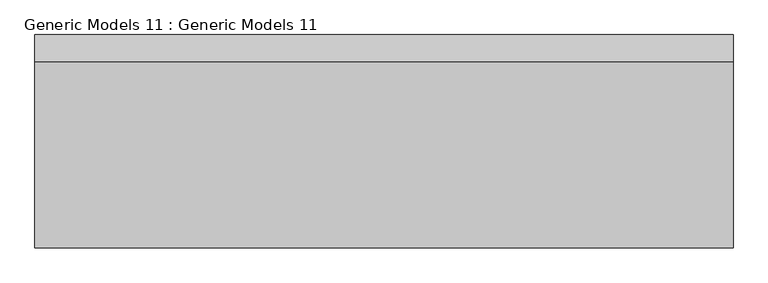
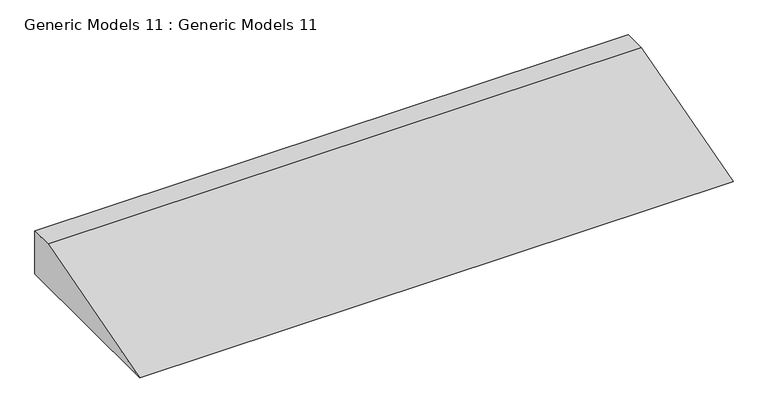
"""IFC4 building model written with IfcOpenShell, lengths in millimetres: proxy geometry, Generic Models 11 : Generic Models 11."""

from ifc_helpers import new_model, si_unit, frame, origin, place, context, project, spatial, polyline, outline, extrude, source, transform, mapped, element, save


def generic_models_11_generic_models_11_be4b57fd(model_context):
    return source(origin(), model_context, "Body", "SweptSolid", [
        extrude(outline(polyline([(3667.2444012, 0.0), (3972.0444012, 0.0), (3972.0444012, -609.6), (2752.8444012, -609.6), (1533.6444012, -609.6), (3667.2444012, 0.0)])), frame((-8482.1519453, 0.0, 0.0), z_axis=(1.0, 0.0, 0.0), x_axis=(0.0, 1.0, 0.0)), (0.0, 0.0, 1.0), 7975.6),
    ])


if __name__ == "__main__":
    model = new_model("IFC4")
    model_context = context("Model", 3, world=origin())
    ifc_project = project(units=[si_unit("LENGTHUNIT", "METRE", prefix="MILLI")], contexts=[model_context])
    site = spatial("IfcSite", under=ifc_project)
    building = spatial("IfcBuilding", under=site)
    placement = place(None, origin())
    generic_models_11_generic_models_11_shape = generic_models_11_generic_models_11_be4b57fd(model_context)
    element("IfcBuildingElementProxy", 1, Name="Generic Models 11 : Generic Models 11", ObjectType="Generic Models 11 : Generic Models 11", at=placement, inside=building, context=model_context, shape_type="MappedRepresentation", body=[
        mapped(generic_models_11_generic_models_11_shape, transform((0.0, 0.0, 0.0), x_axis=(1.0, 0.0, 0.0), y_axis=(0.0, 1.0, 0.0), z_axis=(0.0, 0.0, 1.0))),
    ])
    save(model, "model.ifc")
